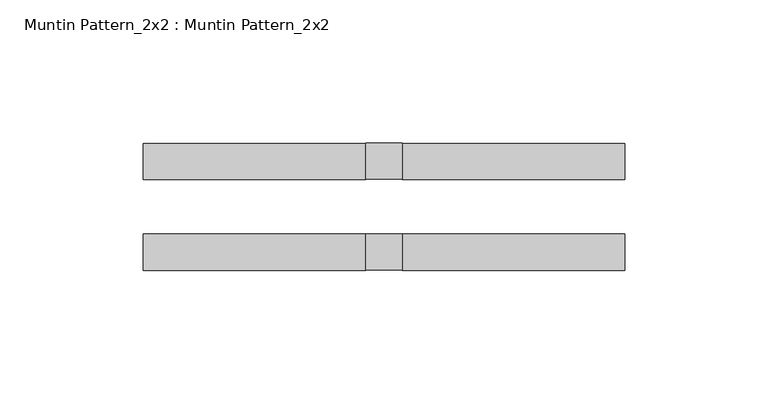
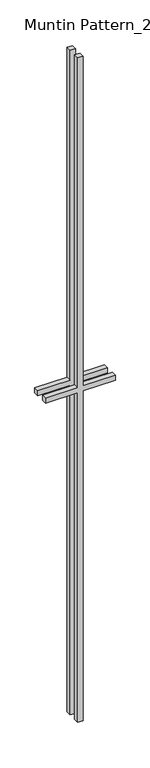
"""IFC4 building model written with IfcOpenShell, lengths in millimetres: proxy geometry, Muntin Pattern_2x2 : Muntin Pattern_2x2."""

from ifc_helpers import new_model, si_unit, frame, origin, place, context, project, spatial, polyline, outline, extrude, source, transform, mapped, element, save


def muntin_pattern_2x2_muntin_pattern_2x2_c5f040ee(model_context):
    return source(origin(), model_context, "Body", "SweptSolid", [
        extrude(outline(polyline([(850.9, -6.35), (850.9, -84.1375), (838.2, -84.1375), (838.2, -6.35), (0.0, -6.35), (0.0, 6.35), (838.2, 6.35), (838.2, 84.1375), (850.9, 84.1375), (850.9, 6.35), (1689.1, 6.35), (1689.1, -6.35), (850.9, -6.35)])), frame((0.0, -22.225, 0.0), z_axis=(0.0, 1.0, 0.0), x_axis=(0.0, 0.0, 1.0)), (0.0, 0.0, 1.0), 12.7),
        extrude(outline(polyline([(850.9, -6.35), (850.9, -84.1375), (838.2, -84.1375), (838.2, -6.35), (0.0, -6.35), (0.0, 6.35), (838.2, 6.35), (838.2, 84.1375), (850.9, 84.1375), (850.9, 6.35), (1689.1, 6.35), (1689.1, -6.35), (850.9, -6.35)])), frame((0.0, 9.525, 0.0), z_axis=(0.0, 1.0, 0.0), x_axis=(0.0, 0.0, 1.0)), (0.0, 0.0, 1.0), 12.7),
    ])


if __name__ == "__main__":
    model = new_model("IFC4")
    model_context = context("Model", 3, world=origin())
    ifc_project = project(units=[si_unit("LENGTHUNIT", "METRE", prefix="MILLI")], contexts=[model_context])
    site = spatial("IfcSite", under=ifc_project)
    building = spatial("IfcBuilding", under=site)
    placement = place(None, origin())
    muntin_pattern_2x2_muntin_pattern_2x2_shape = muntin_pattern_2x2_muntin_pattern_2x2_c5f040ee(model_context)
    element("IfcBuildingElementProxy", 1, Name="Muntin Pattern_2x2 : Muntin Pattern_2x2", ObjectType="Muntin Pattern_2x2 : Muntin Pattern_2x2", at=placement, inside=building, context=model_context, shape_type="MappedRepresentation", body=[
        mapped(muntin_pattern_2x2_muntin_pattern_2x2_shape, transform((0.0, 0.0, 0.0), x_axis=(1.0, 0.0, 0.0), y_axis=(0.0, 1.0, 0.0), z_axis=(0.0, 0.0, 1.0))),
    ])
    save(model, "model.ifc")

# Revit data of these elements
# Type "Muntin Pattern_2x2 : Muntin Pattern_2x2"
#   Width [instance default] = 4' - 0"
#   Thickness = 0' - 0 1/2"
#   Height [instance default] = 4' - 0"
#   Distance = 0' - 0 3/4"
#   Interior Material [instance default] = none
#   Exterior Material [instance default] = none
#   Default Elevation = 0
# Element 1 (IfcBuildingElementProxy, "Muntin Pattern_2x2 : Muntin Pattern_2x2")
#   Width = 0' - 6 5/8"
#   Height = 5' - 6 1/2"
#   Interior Material = Wood - Stained
#   Exterior Material = Clad - White
#   Materials on its faces: "Clad - White", "Wood - Stained"
# Materials
#   "Clad - White": class "Wood", colour RGB 242 242 238, transparency 0, Cost = 0
#   "Wood - Stained": class "Wood", colour RGB 224 178 126, transparency 0, Cost = 0
